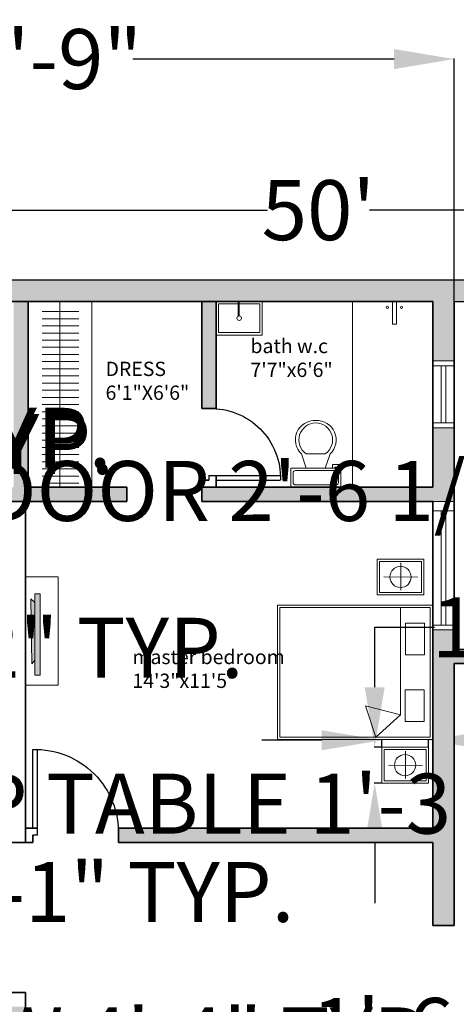
# Model space of a CAD drawing. Units: inches. Extents: x 23 to 3024, y 4 to 1405.
# Tile 3 of 7: x 2375 to 2558, y 992 to 1405. Entities that reach past the tile are written whole.
import ezdxf

# ---------------------------------------------------------------- set-up
doc = ezdxf.new("R2010")
doc.units = ezdxf.units.IN
doc.header["$MEASUREMENT"] = 0
for name, color, linetype, lineweight in [('A-ANNO-DIMS', 2, 'Continuous', 18), ('A-DOOR', 4, 'Continuous', 25), ('A-EQPM', 8, 'Continuous', 18), ('A-EQPM-PATT', 7, 'Continuous', 13), ('A-FLOR-CASE', 9, 'Continuous', 18), ('A-FLOR-FIXT', 9, 'Continuous', 18), ('A-WALL', 7, 'Continuous', 35), ('A-WALL-PATT', 189, 'Continuous', 13), ('C-PROP', 7, 'Continuous', 30)]:
    doc.layers.add(name, color=color, linetype=linetype, lineweight=lineweight)
for name, color, linetype, lineweight, true_color in [('A-AREA-IDEN', 30, 'Continuous', 18, 0xf8991e), ('A-FURN', 141, 'Continuous', 18, 0xadddf7), ('A-GLAZ', 30, 'Continuous', 18, 0xf26722)]:
    doc.layers.add(name, color=color, linetype=linetype, lineweight=lineweight, true_color=true_color)
doc.styles.get("Standard").update_dxf_attribs({"font": 'arial.ttf'})
doc.dimstyles.get("Standard").update_dxf_attribs({"dimtxt": 25.18, "dimasz": 25.18, "dimexe": 0.18, "dimexo": 0.0625, "dimgap": 0.09, "dimtad": 0, "dimtih": 1, "dimtoh": 1, "dimdec": 0, "dimrnd": 10, "dimzin": 0, "dimdsep": 46, "dimlunit": 3, "dimtxsty": 'Standard', "dimcen": 0.09, "dimadec": 0, "dimazin": 0, "dimtfac": 1, "dimtdec": 0, "dimtofl": 0, "dimtmove": 0, "dimatfit": 3, "dimfxl": 1, "dimtolj": 1, "dimtzin": 0, "dimarcsym": 0})

# ---------------------------------------------------------------- blocks, each defined once
blk = doc.blocks.new('*D9')
at = {"layer": 'A-ANNO-DIMS', "color": 0, "lineweight": -2, "transparency": 16777216}
for p, q in [((2200.45, 1295.99), (2200.45, 1325.4)), ((2225.63, 1325.22), (2478.99, 1325.22)), ((2775.27, 1325.22), (2521.91, 1325.22)), ((2800.45, 1295.99), (2800.45, 1325.4))]:
    blk.add_line(p, q, dxfattribs=at)
at = {"layer": 'A-ANNO-DIMS', "color": 0, "transparency": 16777216}
for points in [[(2225.63, 1329.42), (2225.63, 1321.02), (2200.45, 1325.22)], [(2775.27, 1329.42), (2775.27, 1321.02), (2800.45, 1325.22)]]:
    blk.add_solid(points, dxfattribs=at)
at = {"layer": 'Defpoints', "color": 0, "transparency": 16777216}
for p in [(2800.45, 1325.22), (2200.45, 1295.93), (2800.45, 1295.93)]:
    blk.add_point(p, dxfattribs=at)
at = {"layer": 'A-ANNO-DIMS', "color": 0, "transparency": 16777216, "insert": (2500.45, 1325.22), "char_height": 25.18, "attachment_point": 5}
blk.add_mtext("\\A1;50'", dxfattribs=at)
blk = doc.blocks.new('*U2')
for p, q in [((9.5, -6), (9.5, -2)), ((-8, -8.5), (-8, -8)), ((-7, -8), (-7, -9.5)), ((-4, -8), (-6, -14)), ((4, -8), (6, -14)), ((-10, -8.5), (-8, -8.5)), ((-10, -9.5), (-10, -8.5)), ((-7, -9.5), (-10, -9.5)), ((4, -14), (-4, -14))]:
    blk.add_line(p, q)
blk.add_lwpolyline([(10.5, -8), (10.5, 0), (-10.5, 0), (-10.5, -8)], close=True)
for points in [[(-9.5, -2), (-9.5, -6)], [(8.5, -1), (-8.5, -1)], [(-8.5, -7), (8.5, -7)]]:
    blk.add_lwpolyline(points)
for centre, radius, start, end in [((-8.625, -1.875), 0.8839, 81.8699, 188.1301), ((8.625, -1.875), 0.8839, 351.8699, 98.1301), ((-8.625, -6.125), 0.8839, 171.869898, 278.1301), ((8.625, -6.125), 0.8839, 261.8699, 8.1301), ((-0.4772, -19.9188), 8.0953, 133.01722, 273.38), ((0.0374, -19.8731), 7.127, 124.50543, 269.7), ((-0.0373, -19.8731), 7.127, 270.3, 55.4946), ((0.4773, -19.9188), 8.0953, 266.62, 46.9828)]:
    blk.add_arc(centre, radius, start, end)
blk = doc.blocks.new('DOOR-SWING-36IN')
for p, q in [((-1, -1), (-1, 35)), ((1, 2), (1, 35)), ((-1, -1), (1, -1))]:
    blk.add_line(p, q)
blk.add_arc((0, 0), 35.01, 88.3634, 181.6366)
blk = doc.blocks.new('DOOR-SWING-30IN')
for p, q in [((1, 1), (-29, 1)), ((1, 1), (1, -1)), ((-2, -1), (-29, -1))]:
    blk.add_line(p, q)
blk.add_arc((0, 0), 29.02, 88.0251, 181.9749)
blk = doc.blocks.new('WINDOW-24IN')
for p, q in [((9, 28), (0, 28)), ((9, 26), (0, 26)), ((3.5, 2), (3.5, 26)), ((5.5, 2), (5.5, 26)), ((9, 2), (0, 2)), ((9, 0), (0, 0))]:
    blk.add_line(p, q)
blk = doc.blocks.new('NIGHTSTAND-LAMP-LARGE')
for p, q in [((10.01, 13.45), (10.02, 1.97)), ((2.85, 7.51), (17.09, 7.41))]:
    blk.add_line(p, q)
for points in [[(0, 15.02), (19.65, 15.02), (19.65, 0), (0, 0)], [(1, 14.02), (18.65, 14.02), (18.65, 1), (1, 1)]]:
    blk.add_lwpolyline(points, close=True)
blk.add_circle((9.82, 7.51), 4.46)
blk = doc.blocks.new('*D22')
at = {"layer": 'A-ANNO-DIMS', "color": 0, "lineweight": -2, "transparency": 16777216}
for p, q in [((2473.98, 956.88), (2473.98, 982.06)), ((2473.98, 982.06), (2499.16, 982.06)), ((2470.81, 931.7), (2474.16, 931.7)), ((2470.81, 913.26), (2474.16, 913.26)), ((2473.98, 888.08), (2473.98, 862.9))]:
    blk.add_line(p, q, dxfattribs=at)
at = {"layer": 'A-ANNO-DIMS', "color": 0, "transparency": 16777216}
for points in [[(2469.78, 956.88), (2478.17, 956.88), (2473.98, 931.7)], [(2469.78, 888.08), (2478.17, 888.08), (2473.98, 913.26)]]:
    blk.add_solid(points, dxfattribs=at)
at = {"layer": 'Defpoints', "color": 0, "transparency": 16777216}
for p in [(2470.74, 931.7), (2473.98, 931.7), (2470.74, 913.26)]:
    blk.add_point(p, dxfattribs=at)
at = {"layer": 'A-ANNO-DIMS', "color": 0, "transparency": 16777216, "insert": (2604.14, 982.06), "char_height": 25.18, "attachment_point": 5}
blk.add_mtext('\\A1;1\'-6 1/2" TYP.', dxfattribs=at)
blk = doc.blocks.new('*D25')
at = {"layer": 'A-ANNO-DIMS', "color": 0, "lineweight": -2, "transparency": 16777216}
for p, q in [((2273.17, 1211.86), (2273.17, 1207.21)), ((2303.45, 1211.86), (2303.45, 1207.21)), ((2247.99, 1207.39), (2222.81, 1207.39)), ((2328.63, 1207.39), (2353.81, 1207.39))]:
    blk.add_line(p, q, dxfattribs=at)
at = {"layer": 'A-ANNO-DIMS', "color": 0, "transparency": 16777216}
for points in [[(2247.99, 1211.58), (2247.99, 1203.19), (2273.17, 1207.39)], [(2328.63, 1211.58), (2328.63, 1203.19), (2303.45, 1207.39)]]:
    blk.add_solid(points, dxfattribs=at)
at = {"layer": 'Defpoints', "color": 0, "transparency": 16777216}
for p in [(2273.17, 1211.93), (2303.45, 1211.93), (2303.45, 1207.39)]:
    blk.add_point(p, dxfattribs=at)
at = {"layer": 'A-ANNO-DIMS', "color": 0, "transparency": 16777216, "insert": (2517, 1207.39), "char_height": 25.18, "attachment_point": 5}
blk.add_mtext('\\A1;DOOR 2\'-6 1/2" TYP.', dxfattribs=at)
blk = doc.blocks.new('*D26')
at = {"layer": 'A-ANNO-DIMS', "color": 0, "lineweight": -2, "transparency": 16777216}
for p, q in [((2307.99, 1267.38), (2307.99, 1292.56)), ((2303.51, 1242.2), (2308.17, 1242.2)), ((2303.51, 1211.93), (2308.17, 1211.93)), ((2307.99, 1186.75), (2307.99, 1161.57))]:
    blk.add_line(p, q, dxfattribs=at)
at = {"layer": 'A-ANNO-DIMS', "color": 0, "transparency": 16777216}
for points in [[(2303.79, 1267.38), (2312.19, 1267.38), (2307.99, 1242.2)], [(2303.79, 1186.75), (2312.19, 1186.75), (2307.99, 1211.93)]]:
    blk.add_solid(points, dxfattribs=at)
at = {"layer": 'Defpoints', "color": 0, "transparency": 16777216}
for p in [(2303.45, 1242.2), (2307.99, 1242.2), (2303.45, 1211.93)]:
    blk.add_point(p, dxfattribs=at)
at = {"layer": 'A-ANNO-DIMS', "color": 0, "transparency": 16777216, "insert": (2307.99, 1227.07), "char_height": 25.18, "attachment_point": 5}
blk.add_mtext('\\A1;2\'-6 1/2" TYP.', dxfattribs=at)
blk = doc.blocks.new('*D27')
at = {"layer": 'A-ANNO-DIMS', "color": 0, "lineweight": -2, "transparency": 16777216}
for p, q in [((2217.25, 952.93), (2217.25, 978.11)), ((2217.25, 978.11), (2242.43, 978.11)), ((2209.51, 952.93), (2217.43, 952.93)), ((2217.25, 926.11), (2217.25, 927.75)), ((2209.51, 900.93), (2217.43, 900.93))]:
    blk.add_line(p, q, dxfattribs=at)
at = {"layer": 'A-ANNO-DIMS', "color": 0, "transparency": 16777216}
for points in [[(2213.05, 927.75), (2221.45, 927.75), (2217.25, 952.93)], [(2213.05, 926.11), (2221.45, 926.11), (2217.25, 900.93)]]:
    blk.add_solid(points, dxfattribs=at)
at = {"layer": 'Defpoints', "color": 0, "transparency": 16777216}
for p in [(2209.45, 952.93), (2217.25, 952.93), (2209.45, 900.93)]:
    blk.add_point(p, dxfattribs=at)
at = {"layer": 'A-ANNO-DIMS', "color": 0, "transparency": 16777216, "insert": (2401.83, 978.11), "char_height": 25.18, "attachment_point": 5}
blk.add_mtext('\\A1;WINDOW 4\'-4" TYP.', dxfattribs=at)
blk = doc.blocks.new('*D30')
at = {"layer": 'A-ANNO-DIMS', "color": 0, "lineweight": -2, "transparency": 16777216}
for p, q in [((2200.45, 1233.86), (2200.45, 1229.55)), ((2209.45, 1233.86), (2209.45, 1229.55)), ((2175.27, 1229.73), (2150.09, 1229.73)), ((2234.63, 1229.73), (2259.81, 1229.73))]:
    blk.add_line(p, q, dxfattribs=at)
at = {"layer": 'A-ANNO-DIMS', "color": 0, "transparency": 16777216}
for points in [[(2175.27, 1233.92), (2175.27, 1225.53), (2200.45, 1229.73)], [(2234.63, 1233.92), (2234.63, 1225.53), (2209.45, 1229.73)]]:
    blk.add_solid(points, dxfattribs=at)
at = {"layer": 'Defpoints', "color": 0, "transparency": 16777216}
for p in [(2200.45, 1233.93), (2209.45, 1233.93), (2209.45, 1229.73)]:
    blk.add_point(p, dxfattribs=at)
at = {"layer": 'A-ANNO-DIMS', "color": 0, "transparency": 16777216, "insert": (2336.64, 1229.73), "char_height": 25.18, "attachment_point": 5}
blk.add_mtext('\\A1;0\'-9" TYP.', dxfattribs=at)
blk = doc.blocks.new('*D35')
at = {"layer": 'A-ANNO-DIMS', "color": 0, "lineweight": -2, "transparency": 16777216}
for p, q in [((2297.24, 975.85), (2297.24, 973.72)), ((2310.67, 975.85), (2310.67, 973.72)), ((2272.06, 973.9), (2246.88, 973.9)), ((2335.85, 973.9), (2361.03, 973.9))]:
    blk.add_line(p, q, dxfattribs=at)
at = {"layer": 'A-ANNO-DIMS', "color": 0, "transparency": 16777216}
for points in [[(2272.06, 978.09), (2272.06, 969.7), (2297.24, 973.9)], [(2335.85, 978.09), (2335.85, 969.7), (2310.67, 973.9)]]:
    blk.add_solid(points, dxfattribs=at)
at = {"layer": 'Defpoints', "color": 0, "transparency": 16777216}
for p in [(2297.24, 975.91), (2310.67, 975.91), (2310.67, 973.9)]:
    blk.add_point(p, dxfattribs=at)
at = {"layer": 'A-ANNO-DIMS', "color": 0, "transparency": 16777216, "insert": (2585.8, 973.9), "char_height": 25.18, "attachment_point": 5}
blk.add_mtext('\\A1;NIGHTSTAND 1\'-1 1/2" TYP.', dxfattribs=at)
blk = doc.blocks.new('*D36')
at = {"layer": 'A-ANNO-DIMS', "color": 0, "lineweight": -2, "transparency": 16777216}
for p, q in [((2312.68, 1013.98), (2312.68, 1039.16)), ((2312.68, 1039.16), (2337.86, 1039.16)), ((2310.73, 988.8), (2312.86, 988.8)), ((2310.73, 975.91), (2312.86, 975.91)), ((2312.68, 950.73), (2312.68, 925.55))]:
    blk.add_line(p, q, dxfattribs=at)
at = {"layer": 'A-ANNO-DIMS', "color": 0, "transparency": 16777216}
for points in [[(2308.48, 1013.98), (2316.88, 1013.98), (2312.68, 988.8)], [(2308.48, 950.73), (2316.88, 950.73), (2312.68, 975.91)]]:
    blk.add_solid(points, dxfattribs=at)
at = {"layer": 'Defpoints', "color": 0, "transparency": 16777216}
for p in [(2310.67, 988.8), (2312.68, 988.8), (2310.67, 975.91)]:
    blk.add_point(p, dxfattribs=at)
at = {"layer": 'A-ANNO-DIMS', "color": 0, "transparency": 16777216, "insert": (2413.51, 1039.16), "char_height": 25.18, "attachment_point": 5}
blk.add_mtext('\\A1;1\'-1" TYP.', dxfattribs=at)
blk = doc.blocks.new('*D37')
at = {"layer": 'A-ANNO-DIMS', "color": 0, "lineweight": -2, "transparency": 16777216}
for p, q in [((2214.42, 1078.46), (2214.42, 1076)), ((2230.01, 1078.46), (2230.01, 1076)), ((2189.24, 1076.18), (2164.06, 1076.18)), ((2255.19, 1076.18), (2280.37, 1076.18))]:
    blk.add_line(p, q, dxfattribs=at)
at = {"layer": 'A-ANNO-DIMS', "color": 0, "transparency": 16777216}
for points in [[(2189.24, 1080.38), (2189.24, 1071.99), (2214.42, 1076.18)], [(2255.19, 1080.38), (2255.19, 1071.99), (2230.01, 1076.18)]]:
    blk.add_solid(points, dxfattribs=at)
at = {"layer": 'Defpoints', "color": 0, "transparency": 16777216}
for p in [(2214.42, 1078.52), (2230.01, 1078.52), (2230.01, 1076.18)]:
    blk.add_point(p, dxfattribs=at)
at = {"layer": 'A-ANNO-DIMS', "color": 0, "transparency": 16777216, "insert": (2499.37, 1076.18), "char_height": 25.18, "attachment_point": 5}
blk.add_mtext('\\A1;LAMP TABLE 1\'-3 1/2" TYP.', dxfattribs=at)
blk = doc.blocks.new('*D38')
at = {"layer": 'A-ANNO-DIMS', "color": 0, "lineweight": -2, "transparency": 16777216}
for p, q in [((2232.35, 1116.41), (2232.35, 1141.59)), ((2232.35, 1141.59), (2257.53, 1141.59)), ((2230.07, 1091.23), (2232.53, 1091.23)), ((2230.07, 1078.52), (2232.53, 1078.52)), ((2232.35, 1053.34), (2232.35, 1028.16))]:
    blk.add_line(p, q, dxfattribs=at)
at = {"layer": 'A-ANNO-DIMS', "color": 0, "transparency": 16777216}
for points in [[(2228.15, 1116.41), (2236.54, 1116.41), (2232.35, 1091.23)], [(2228.15, 1053.34), (2236.54, 1053.34), (2232.35, 1078.52)]]:
    blk.add_solid(points, dxfattribs=at)
at = {"layer": 'Defpoints', "color": 0, "transparency": 16777216}
for p in [(2230.01, 1091.23), (2232.35, 1091.23), (2230.01, 1078.52)]:
    blk.add_point(p, dxfattribs=at)
at = {"layer": 'A-ANNO-DIMS', "color": 0, "transparency": 16777216, "insert": (2362.51, 1141.59), "char_height": 25.18, "attachment_point": 5}
blk.add_mtext('\\A1;1\'-0 1/2" TYP.', dxfattribs=at)
blk = doc.blocks.new('*D39')
at = {"layer": 'A-ANNO-DIMS', "color": 0, "lineweight": -2, "transparency": 16777216}
for p, q in [((2501.85, 1102.79), (2476.67, 1102.79)), ((2527.03, 1099.9), (2527.03, 1102.97)), ((2546.68, 1099.9), (2546.68, 1102.97)), ((2571.86, 1102.79), (2597.04, 1102.79))]:
    blk.add_line(p, q, dxfattribs=at)
at = {"layer": 'A-ANNO-DIMS', "color": 0, "transparency": 16777216}
for points in [[(2501.85, 1106.99), (2501.85, 1098.59), (2527.03, 1102.79)], [(2571.86, 1106.99), (2571.86, 1098.59), (2546.68, 1102.79)]]:
    blk.add_solid(points, dxfattribs=at)
at = {"layer": 'Defpoints', "color": 0, "transparency": 16777216}
for p in [(2527.03, 1099.84), (2546.68, 1102.79), (2546.68, 1099.84)]:
    blk.add_point(p, dxfattribs=at)
at = {"layer": 'A-ANNO-DIMS', "color": 0, "transparency": 16777216, "insert": (2816.04, 1102.79), "char_height": 25.18, "attachment_point": 5}
blk.add_mtext('\\A1;LAMP TABLE 1\'-7 1/2" TYP.', dxfattribs=at)
blk = doc.blocks.new('*D40')
at = {"layer": 'A-ANNO-DIMS', "color": 0, "lineweight": -2, "transparency": 16777216}
for p, q in [((2524.09, 1125.02), (2524.09, 1150.2)), ((2524.09, 1150.2), (2549.27, 1150.2)), ((2526.97, 1099.84), (2523.91, 1099.84)), ((2526.97, 1084.82), (2523.91, 1084.82)), ((2524.09, 1059.64), (2524.09, 1034.46))]:
    blk.add_line(p, q, dxfattribs=at)
at = {"layer": 'A-ANNO-DIMS', "color": 0, "transparency": 16777216}
for points in [[(2519.89, 1125.02), (2528.28, 1125.02), (2524.09, 1099.84)], [(2519.89, 1059.64), (2528.28, 1059.64), (2524.09, 1084.82)]]:
    blk.add_solid(points, dxfattribs=at)
at = {"layer": 'Defpoints', "color": 0, "transparency": 16777216}
for p in [(2524.09, 1099.84), (2527.03, 1099.84), (2527.03, 1084.82)]:
    blk.add_point(p, dxfattribs=at)
at = {"layer": 'A-ANNO-DIMS', "color": 0, "transparency": 16777216, "insert": (2624.91, 1150.2), "char_height": 25.18, "attachment_point": 5}
blk.add_mtext('\\A1;1\'-3" TYP.', dxfattribs=at)
blk = doc.blocks.new('*D44')
at = {"layer": 'A-ANNO-DIMS', "color": 0, "lineweight": -2, "transparency": 16777216}
for p, q in [((2200.45, 1295.99), (2200.45, 1388.79)), ((2225.63, 1388.61), (2335.4, 1388.61)), ((2532.27, 1388.61), (2422.5, 1388.61)), ((2557.45, 1286.99), (2557.45, 1388.79))]:
    blk.add_line(p, q, dxfattribs=at)
at = {"layer": 'A-ANNO-DIMS', "color": 0, "transparency": 16777216}
for points in [[(2225.63, 1392.81), (2225.63, 1384.42), (2200.45, 1388.61)], [(2532.27, 1392.81), (2532.27, 1384.42), (2557.45, 1388.61)]]:
    blk.add_solid(points, dxfattribs=at)
at = {"layer": 'Defpoints', "color": 0, "transparency": 16777216}
for p in [(2557.45, 1388.61), (2200.45, 1295.93), (2557.45, 1286.93)]:
    blk.add_point(p, dxfattribs=at)
at = {"layer": 'A-ANNO-DIMS', "color": 0, "transparency": 16777216, "insert": (2378.95, 1388.61), "char_height": 25.18, "attachment_point": 5}
blk.add_mtext('\\A1;29\'-9"', dxfattribs=at)

msp = doc.modelspace()

# ---------------------------------------------------------------- hatches: boundary and pattern name
at = {"layer": 'A-EQPM-PATT'}
h = msp.add_hatch(color=256, dxfattribs=at)
h.dxf.hatch_style = 1
h.paths.add_polyline_path([(2566.39, 889.19), (2562.89, 889.19), (2562.89, 848.35), (2566.39, 848.35)])
h.paths.add_polyline_path([(2562.89, 883.28), (2559.32, 885.34), (2559.32, 851.44), (2562.89, 854.81)])
h.paths.add_polyline_path([(2370.36, 1159.16), (2369.43, 1157.81), (2369.43, 1135.58), (2370.36, 1134.43)])
h.paths.add_polyline_path([(2369.43, 1162.31), (2367.73, 1162.31), (2367.73, 1131.3), (2369.43, 1131.3)])
h.paths.add_polyline_path([(2381.34, 1160.62), (2379.7, 1162.16), (2380.08, 1134.79), (2381.34, 1136.43)])
h.paths.add_polyline_path([(2383.55, 1164.18), (2381.34, 1164.18), (2381.34, 1130.16), (2383.55, 1130.16)])
at = {"layer": 'A-WALL-PATT'}
h = msp.add_hatch(color=256, dxfattribs=at)
h.dxf.hatch_style = 1
h.paths.add_polyline_path([(2209.45, 1233.93), (2200.45, 1233.93), (2200.45, 1160.43), (2209.45, 1160.43), (2209.45, 1167.77), (2209.45, 1202.93), (2306.45, 1202.93), (2306.45, 1208.93), (2300.45, 1208.93), (2209.45, 1208.93)], flags=17)
h.paths.add_polyline_path([(2800.45, 1295.93), (2200.45, 1295.93), (2160.45, 1295.93), (2160.45, 575.93), (2200.45, 575.93), (2228.06, 575.93), (2228.06, 584.93), (2209.45, 584.93), (2209.45, 856.93), (2200.45, 856.93), (2200.45, 581.93), (2166.45, 581.93), (2166.45, 1289.93), (2200.45, 1289.93), (2200.45, 1261.93), (2209.45, 1261.93), (2209.45, 1286.93), (2244.45, 1286.93), (2300.45, 1286.93), (2300.45, 1241.93), (2301.45, 1241.93, -0.017236), (2303.45, 1241.93), (2306.45, 1241.93), (2306.45, 1286.93), (2548.45, 1286.93), (2548.45, 1261.93), (2557.45, 1261.93), (2557.45, 1286.93), (2791.45, 1286.93), (2791.45, 1140.93), (2613.74, 1140.93), (2613.74, 1134.93), (2791.45, 1134.93), (2791.45, 927.1), (2800.45, 927.1)])
h.paths.add_polyline_path([(2166.06, 1284.53), (2166.03, 1284.87), (2166.29, 1284.91), (2166.32, 1284.58)], flags=16)
h.paths.add_polyline_path([(2557.45, 1233.93), (2548.45, 1233.93), (2548.45, 1208.93), (2514.78, 1208.93), (2457.45, 1208.93), (2451.45, 1208.93), (2451.45, 1202.93), (2548.45, 1202.93), (2557.45, 1202.93)], flags=17)
h.paths.add_polyline_path([(2457.45, 1286.93), (2451.45, 1286.93), (2451.45, 1241.93), (2454.45, 1241.93, -0.017236), (2456.45, 1241.93), (2457.45, 1241.93)], flags=17)
h.paths.add_polyline_path([(2419.96, 1208.93), (2378.45, 1208.93), (2378.45, 1286.93), (2372.45, 1286.93), (2372.45, 1208.93), (2352.45, 1208.93), (2352.45, 1202.93), (2419.96, 1202.93)], flags=17)
h.paths.add_polyline_path([(2557.45, 1134.93), (2563.84, 1134.93), (2563.84, 1140.93), (2557.45, 1140.93), (2557.45, 1149.12), (2548.45, 1149.12), (2548.45, 1103.07), (2548.45, 1065.93), (2416.45, 1065.93), (2416.45, 1064.93, -0.014283), (2416.45, 1062.93), (2416.45, 1059.93), (2548.45, 1059.93), (2548.45, 1025.12), (2557.45, 1025.12)], flags=17)
h.paths.add_polyline_path([(2332.45, 1062.93, -0.014283), (2332.45, 1064.93), (2332.45, 1065.93), (2209.45, 1065.93), (2209.45, 1108.43), (2200.45, 1108.43), (2200.45, 1042.43), (2209.45, 1042.43), (2209.45, 1059.93), (2332.45, 1059.93)], flags=17)
h.paths.add_polyline_path([(2332.45, 996.93), (2209.45, 996.93), (2209.45, 1014.43), (2200.45, 1014.43), (2200.45, 952.93), (2209.45, 952.93), (2209.45, 990.93), (2332.45, 990.93), (2332.45, 991.93, -0.014283), (2332.45, 993.93)], flags=17)
h.paths.add_polyline_path([(2209.45, 900.93), (2200.45, 900.93), (2200.45, 856.93), (2209.45, 856.93), (2255.95, 856.93), (2255.95, 862.93), (2209.45, 862.93)], flags=17)
h.paths.add_polyline_path([(2377.45, 823.93), (2374.45, 823.93, -0.017236), (2372.45, 823.93), (2371.45, 823.93), (2371.45, 763.93), (2312.45, 763.93), (2312.45, 791.27), (2312.45, 796.43), (2306.45, 796.43), (2306.45, 757.93), (2436.95, 757.93), (2436.95, 763.93), (2377.45, 763.93)], flags=17)
h.paths.add_polyline_path([(2557.45, 948.81), (2548.45, 948.81), (2548.45, 763.93), (2488.95, 763.93), (2488.95, 757.93), (2560.45, 757.93), (2560.45, 760.93), (2562.45, 760.93), (2562.45, 763.93), (2557.45, 763.93)], flags=17)
h.paths.add_polyline_path([(2377.45, 990.93), (2371.45, 990.93), (2371.45, 862.93), (2306.45, 862.93), (2306.45, 856.93), (2306.45, 824.43), (2312.45, 824.43), (2312.45, 856.93), (2371.45, 856.93), (2377.45, 856.93)], flags=17)
h.paths.add_polyline_path([(2800.45, 875.1), (2791.45, 875.1), (2791.45, 763.93), (2719.93, 763.93), (2719.93, 757.93), (2791.45, 757.93), (2791.45, 584.93), (2338.88, 584.93), (2338.88, 575.93), (2800.45, 575.93)], flags=17)
h.paths.add_polyline_path([(2667.93, 763.93), (2596.45, 763.93), (2596.45, 762.93, -0.014283), (2596.45, 760.93), (2596.45, 757.93), (2667.93, 757.93)], flags=16)

# ---------------------------------------------------------------- linework, layer by layer
at = {"layer": 'A-EQPM'}
for p, q in [((2381.34, 1160.62), (2379.7, 1162.16)), ((2379.7, 1162.16), (2380.08, 1134.79)), ((2380.08, 1134.79), (2381.34, 1136.43))]:
    msp.add_line(p, q, dxfattribs=at)
for points in [[(2377.45, 1171.33), (2391.17, 1171.33), (2391.17, 1125.86), (2377.45, 1125.86)], [(2383.55, 1164.18), (2381.34, 1164.18), (2381.34, 1130.16), (2383.55, 1130.16)]]:
    msp.add_lwpolyline(points, close=True, dxfattribs=at)
at = {"layer": 'A-FLOR-CASE'}
for p, q in [((2391.85, 1286.93), (2391.85, 1208.93)), ((2384.46, 1282.66), (2399.78, 1282.66)), ((2384.46, 1279.66), (2399.78, 1279.66)), ((2384.46, 1276.66), (2399.78, 1276.66)), ((2384.46, 1273.66), (2399.78, 1273.66)), ((2384.46, 1270.66), (2399.78, 1270.66)), ((2384.46, 1267.66), (2399.78, 1267.66)), ((2384.46, 1264.66), (2399.78, 1264.66)), ((2384.46, 1261.66), (2399.78, 1261.66)), ((2384.46, 1258.66), (2399.78, 1258.66)), ((2384.46, 1255.66), (2399.78, 1255.66)), ((2384.46, 1252.66), (2399.78, 1252.66)), ((2384.46, 1249.66), (2399.78, 1249.66)), ((2384.46, 1246.66), (2399.78, 1246.66)), ((2384.46, 1243.66), (2399.78, 1243.66)), ((2384.46, 1240.66), (2399.78, 1240.66)), ((2384.46, 1237.66), (2399.78, 1237.66)), ((2384.46, 1234.66), (2399.78, 1234.66)), ((2384.46, 1231.66), (2399.78, 1231.66)), ((2384.46, 1228.66), (2399.78, 1228.66)), ((2384.46, 1225.66), (2399.78, 1225.66)), ((2384.46, 1222.66), (2399.78, 1222.66)), ((2384.46, 1219.66), (2399.78, 1219.66)), ((2384.46, 1216.66), (2399.78, 1216.66)), ((2384.46, 1213.66), (2399.78, 1213.66)), ((2384.46, 1210.66), (2399.78, 1210.66))]:
    msp.add_line(p, q, dxfattribs=at)
msp.add_lwpolyline([(2378.45, 1286.93), (2405.26, 1286.93), (2405.26, 1208.93), (2378.45, 1208.93)], close=True, dxfattribs=at)
at = {"layer": 'A-FLOR-FIXT'}
for points in [[(2457.45, 1286.93), (2476.83, 1286.93), (2476.83, 1272.83), (2457.45, 1272.83)], [(2458.45, 1285.93), (2475.83, 1285.93), (2475.83, 1273.83), (2458.45, 1273.83)], [(2467.14, 1286.93), (2466.71, 1286.93), (2466.71, 1280.74), (2467.14, 1280.74)], [(2548.45, 1286.93), (2514.78, 1286.93), (2514.78, 1208.93), (2548.45, 1208.93)], [(2531.62, 1286.93), (2533.19, 1286.93), (2533.19, 1277.38), (2531.62, 1277.38)]]:
    msp.add_lwpolyline(points, close=True, dxfattribs=at)
for centre, radius in [((2529.39, 1284.47), 0.471), ((2535.35, 1284.47), 0.471), ((2467.14, 1279.88), 0.96)]:
    msp.add_circle(centre, radius, dxfattribs=at)
at = {"layer": 'A-FURN'}
for p, q in [((2534.97, 1158.47), (2534.97, 1113.43)), ((2524.54, 1104.07), (2520.17, 1117.27)), ((2520.17, 1117.27), (2534.97, 1113.43)), ((2534.97, 1113.43), (2524.54, 1104.07))]:
    msp.add_line(p, q, dxfattribs=at)
for points in [[(2548.45, 1159.47), (2483.29, 1159.47), (2483.29, 1103.07), (2548.45, 1103.07)], [(2547.45, 1158.47), (2484.29, 1158.47), (2484.29, 1104.07), (2547.45, 1104.07)], [(2537.08, 1151.93), (2544.98, 1151.93), (2544.98, 1138.61), (2537.08, 1138.61)], [(2536.94, 1123.99), (2544.84, 1123.99), (2544.84, 1110.67), (2536.94, 1110.67)]]:
    msp.add_lwpolyline(points, close=True, dxfattribs=at)
at = {"layer": 'A-GLAZ'}
for p, q in [((2548.45, 1202.93), (2557.45, 1202.93)), ((2557.45, 1199.12), (2548.45, 1199.12)), ((2551.95, 1199.12), (2551.95, 1151.12)), ((2553.95, 1199.12), (2553.95, 1151.12)), ((2557.45, 1151.12), (2548.45, 1151.12)), ((2557.45, 1149.12), (2548.45, 1149.12))]:
    msp.add_line(p, q, dxfattribs=at)
at = {"layer": 'A-WALL'}
for p, q in [((2306.45, 1286.93), (2548.45, 1286.93)), ((2378.45, 1208.93), (2378.45, 1286.93)), ((2451.45, 1241.93), (2451.45, 1286.93)), ((2457.45, 1241.88), (2457.45, 1286.93)), ((2548.45, 1208.93), (2548.45, 1286.93)), ((2557.45, 1140.93), (2557.45, 1286.93)), ((2457.45, 1241.93), (2451.45, 1241.93)), ((2451.45, 1208.93), (2451.45, 1211.93)), ((2454.45, 1211.93), (2451.45, 1211.93)), ((2457.45, 1208.93), (2457.45, 1213.93)), ((2378.45, 1208.93), (2419.96, 1208.93)), ((2419.96, 1208.93), (2419.96, 1202.93)), ((2451.45, 1208.93), (2451.45, 1202.93)), ((2457.45, 1208.93), (2451.45, 1208.93)), ((2457.45, 1208.93), (2548.45, 1208.93)), ((2352.45, 1202.93), (2419.96, 1202.93)), ((2377.45, 1065.93), (2377.45, 1202.93)), ((2451.45, 1202.93), (2548.45, 1202.93)), ((2548.45, 1065.93), (2548.45, 1202.93)), ((2557.45, 1140.93), (2791.45, 1140.93)), ((2557.45, 1134.93), (2791.45, 1134.93)), ((2557.45, 1134.93), (2557.45, 1025.12)), ((2377.45, 1065.93), (2382.45, 1065.93)), ((2377.45, 1065.93), (2377.45, 1059.93)), ((2416.41, 1065.93), (2548.45, 1065.93)), ((2416.45, 1065.93), (2416.45, 1059.93)), ((2380.45, 1062.93), (2380.45, 1059.93)), ((2368.45, 1059.93), (2380.45, 1059.93)), ((2416.45, 1059.93), (2548.45, 1059.93)), ((2548.45, 1059.93), (2548.45, 1025.12)), ((2548.45, 1025.12), (2557.45, 1025.12)), ((2368.45, 996.93), (2377.45, 996.93)), ((2377.45, 996.93), (2377.45, 856.93))]:
    msp.add_line(p, q, dxfattribs=at)
at = {"layer": 'C-PROP'}
for p, q in [((2200.45, 1295.93), (2800.45, 1295.93)), ((2557.45, 1286.93), (2791.45, 1286.93))]:
    msp.add_line(p, q, dxfattribs=at)

# ---------------------------------------------------------------- block references
at = {"layer": 'A-DOOR', "extrusion": (0, 0, -1), "zscale": -1}
for name, p in [('DOOR-SWING-30IN', (-2455.45, 1212.93)), ('DOOR-SWING-36IN', (-2381.45, 1063.93))]:
    msp.add_blockref(name, p, dxfattribs=at)
at = {"layer": 'A-FLOR-FIXT', "rotation": 180}
msp.add_blockref('*U2', (2499.32, 1208.93), dxfattribs=at)
at = {"layer": 'A-FURN'}
for p in [(2525.12, 1163.82), (2527.03, 1084.82)]:
    msp.add_blockref('NIGHTSTAND-LAMP-LARGE', p, dxfattribs=at)
at = {"layer": 'A-GLAZ'}
msp.add_blockref('WINDOW-24IN', (2548.45, 1233.93), dxfattribs=at)

# ---------------------------------------------------------------- texts
at = {"layer": 'A-AREA-IDEN', "char_height": 6, "attachment_point": 1}
for s, width, insert in [('bath w.c\\P7\'7"x6\'6" ', 46.8839, (2471.89, 1271.22)), ('DRESS\\P6\'1"X6\'6"', 46.8839, (2411.02, 1261.62)), ('master bedroom\\P14\'3"x11\'5"', 65.3165, (2422.31, 1140.74))]:
    msp.add_mtext_dynamic_manual_height_columns(s, width=width, gutter_width=1, heights=[0], dxfattribs=dict(at, insert=insert))

# ---------------------------------------------------------------- dimensions: what is measured, and where the dimension line sits
at = {"layer": 'A-ANNO-DIMS'}
for base, p2, override, picture, middle in [((2557.45, 1388.61), (2557.45, 1286.93), {"dimdec": 1, "dimlfac": 1, "dimrnd": 0, "dimzin": 1, "dimdsep": 46, "dimlunit": 4, "dimfrac": 2}, '*D44', (2378.95, 1388.61)), ((2800.45, 1325.22), (2800.45, 1295.93), {"dimclrd": 0, "dimclre": 0, "dimclrt": 0}, '*D9', (2500.45, 1325.22))]:
    dim = msp.add_linear_dim(base=base, p1=(2200.45, 1295.93), p2=p2, dimstyle='Standard', override=override, dxfattribs=at)
    dim.commit()
    dim.dimension.update_dxf_attribs({"geometry": picture, "text_midpoint": middle})
for base, p1, p2, text, picture, middle in [((2307.99, 1242.2), (2303.45, 1211.93), (2303.45, 1242.2), '<> TYP.', '*D26', (2307.99, 1227.07)), ((2232.35, 1091.23), (2230.01, 1078.52), (2230.01, 1091.23), '<> TYP.', '*D38', (2362.51, 1141.59)), ((2524.09, 1099.84), (2527.03, 1084.82), (2527.03, 1099.84), '<> TYP.', '*D40', (2624.91, 1150.2)), ((2312.68, 988.8), (2310.67, 975.91), (2310.67, 988.8), '<> TYP.', '*D36', (2413.51, 1039.16)), ((2473.98, 931.7), (2470.74, 913.26), (2470.74, 931.7), '<> TYP.', '*D22', (2604.14, 982.06)), ((2217.25, 952.93), (2209.45, 900.93), (2209.45, 952.93), 'WINDOW <> TYP.', '*D27', (2401.83, 978.11))]:
    dim = msp.add_linear_dim(base=base, p1=p1, p2=p2, angle=90, text=text, dimstyle='Standard', override={"dimdec": 1, "dimlfac": 1, "dimrnd": 0, "dimzin": 1, "dimdsep": 46, "dimlunit": 4, "dimfrac": 2}, dxfattribs=at)
    dim.commit()
    dim.dimension.update_dxf_attribs({"geometry": picture, "text_midpoint": middle})
for base, p1, p2, text, picture, middle in [((2303.45, 1207.39), (2273.17, 1211.93), (2303.45, 1211.93), 'DOOR <> TYP.', '*D25', (2517, 1207.39)), ((2209.45, 1229.73), (2200.45, 1233.93), (2209.45, 1233.93), '<> TYP.', '*D30', (2336.64, 1229.73)), ((2546.6795, 1102.7891), (2527.0344, 1099.8423), (2546.6795, 1099.8423), 'LAMP TABLE <> TYP.', '*D39', (2816.0374, 1102.7891)), ((2230.01, 1076.18), (2214.42, 1078.52), (2230.01, 1078.52), 'LAMP TABLE <> TYP.', '*D37', (2499.37, 1076.18)), ((2310.67, 973.9), (2297.24, 975.91), (2310.67, 975.91), 'NIGHTSTAND <> TYP.', '*D35', (2585.8, 973.9))]:
    dim = msp.add_linear_dim(base=base, p1=p1, p2=p2, text=text, dimstyle='Standard', override={"dimdec": 1, "dimlfac": 1, "dimrnd": 0, "dimzin": 1, "dimdsep": 46, "dimlunit": 4, "dimfrac": 2}, dxfattribs=at)
    dim.commit()
    dim.dimension.update_dxf_attribs({"geometry": picture, "text_midpoint": middle})

doc.saveas('drawing.dxf')
